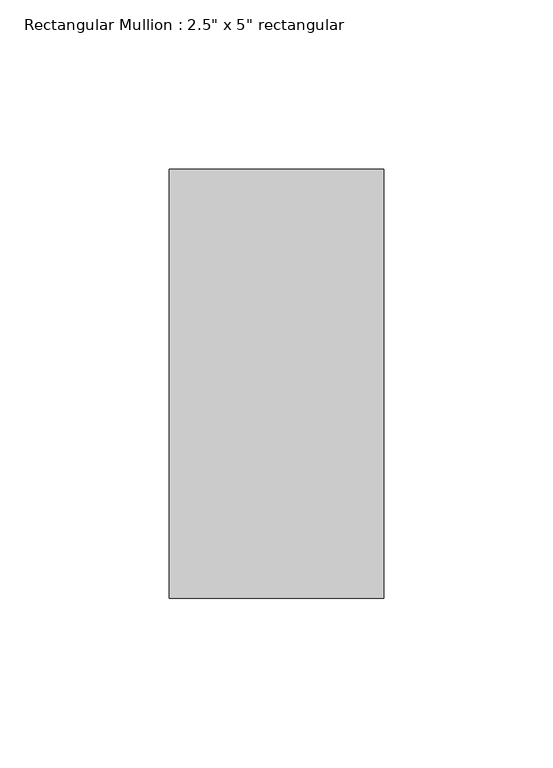
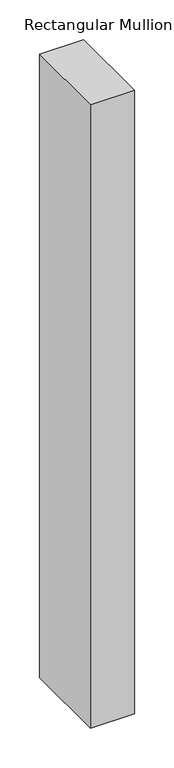
"""IFC4 building model written with IfcOpenShell, lengths in millimetres: member geometry."""

from ifc_helpers import new_model, si_unit, frame, origin, place, context, project, spatial, polyline, outline, extrude, source, transform, mapped, element, save


def member_3f9fbe84(model_context):
    return source(origin(), model_context, "Body", "SweptSolid", [
        extrude(outline(polyline([(0.0, 63.5), (0.0, -63.5), (-63.5, -63.5), (-63.5, 63.5), (0.0, 63.5)])), frame((0.0, 0.0, -952.6412675), z_axis=(0.0, 0.0, 1.0), x_axis=(1.0, 0.0, 0.0)), (0.0, 0.0, 1.0), 952.6412675),
    ])


if __name__ == "__main__":
    model = new_model("IFC4")
    model_context = context("Model", 3, world=origin())
    ifc_project = project(units=[si_unit("LENGTHUNIT", "METRE", prefix="MILLI")], contexts=[model_context])
    site = spatial("IfcSite", under=ifc_project)
    building = spatial("IfcBuilding", under=site)
    placement = place(None, origin())
    member_shape = member_3f9fbe84(model_context)
    element("IfcMember", 1, ObjectType="Rectangular Mullion : 2.5\" x 5\" rectangular", at=placement, inside=building, context=model_context, shape_type="MappedRepresentation", body=[
        mapped(member_shape, transform((0.0, 0.0, 0.0), x_axis=(1.0, 0.0, 0.0), y_axis=(0.0, 1.0, 0.0), z_axis=(0.0, 0.0, 1.0))),
    ])
    save(model, "model.ifc")

# Revit data of these elements
# Type "Rectangular Mullion : 2.5\" x 5\" rectangular"
#   built-in parameter 1007304 = 0.416667 (stored number, unit not read)
#   built-in parameter 1007301 = 0.104167 (stored number, unit not read)
#   built-in parameter 1007300 = 0.104167 (stored number, unit not read)
# Element 1 (IfcMember, "Rectangular Mullion : 2.5\" x 5\" rectangular")
#   Materials on its faces: "Aluminum"
# Materials
#   "Aluminum": class "Metal", colour RGB 247 247 247, transparency 0, Description = "Aluminum 6061", Cost = 0
